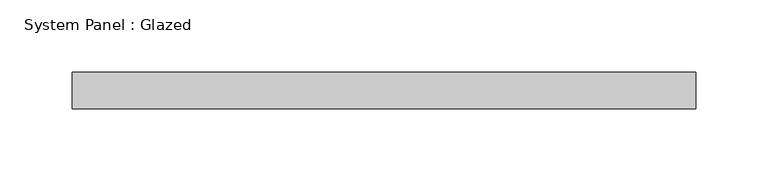
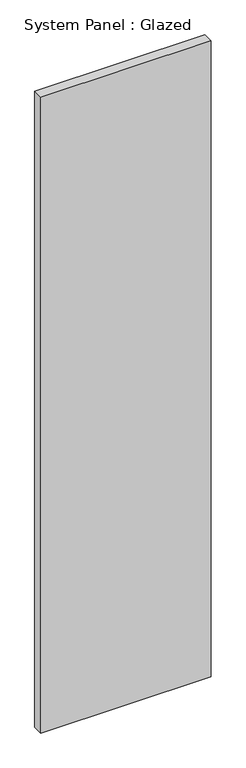
"""IFC4 building model written with IfcOpenShell, lengths in millimetres: plate geometry, System Panel : Glazed."""

from ifc_helpers import new_model, si_unit, origin, origin_with_axes, place, context, project, spatial, polyline, outline, extrude, source, transform, mapped, element, save


def system_panel_glazed_19c201ce(model_context):
    return source(origin(), model_context, "Body", "SweptSolid", [
        extrude(outline(polyline([(215.9, 19.05), (-215.9, 19.05), (-215.9, 44.45), (215.9, 44.45), (215.9, 19.05)])), origin_with_axes(), (0.0, 0.0, 1.0), 1701.8),
    ])


if __name__ == "__main__":
    model = new_model("IFC4")
    model_context = context("Model", 3, world=origin())
    ifc_project = project(units=[si_unit("LENGTHUNIT", "METRE", prefix="MILLI")], contexts=[model_context])
    site = spatial("IfcSite", under=ifc_project)
    building = spatial("IfcBuilding", under=site)
    placement = place(None, origin())
    system_panel_glazed_shape = system_panel_glazed_19c201ce(model_context)
    element("IfcPlate", 1, ObjectType="System Panel : Glazed", at=placement, inside=building, context=model_context, shape_type="MappedRepresentation", body=[
        mapped(system_panel_glazed_shape, transform((0.0, 0.0, 0.0), x_axis=(1.0, 0.0, 0.0), y_axis=(0.0, 1.0, 0.0), z_axis=(0.0, 0.0, 1.0))),
    ])
    save(model, "model.ifc")

# Revit data of these elements
# Type "System Panel : Glazed"
#   Construction Type Id = "GSP4R"
#   Analytic Construction = "1/8 in Pilkington single glazing"
#   Visual Light Transmittance = 0.9
#   Solar Heat Gain Coefficient = 0.86
#   Heat Transfer Coefficient (U) = 1.18115 BTU/(h·ft²·°F)
#   Define Thermal Properties by = 1
# Element 1 (IfcPlate, "System Panel : Glazed")
#   Materials on its faces: "Glass"
# Materials
#   "Glass": class "Glass", colour RGB 0 128 192, transparency 0.75, Description = "Soda Lime Glass", Cost = 0
